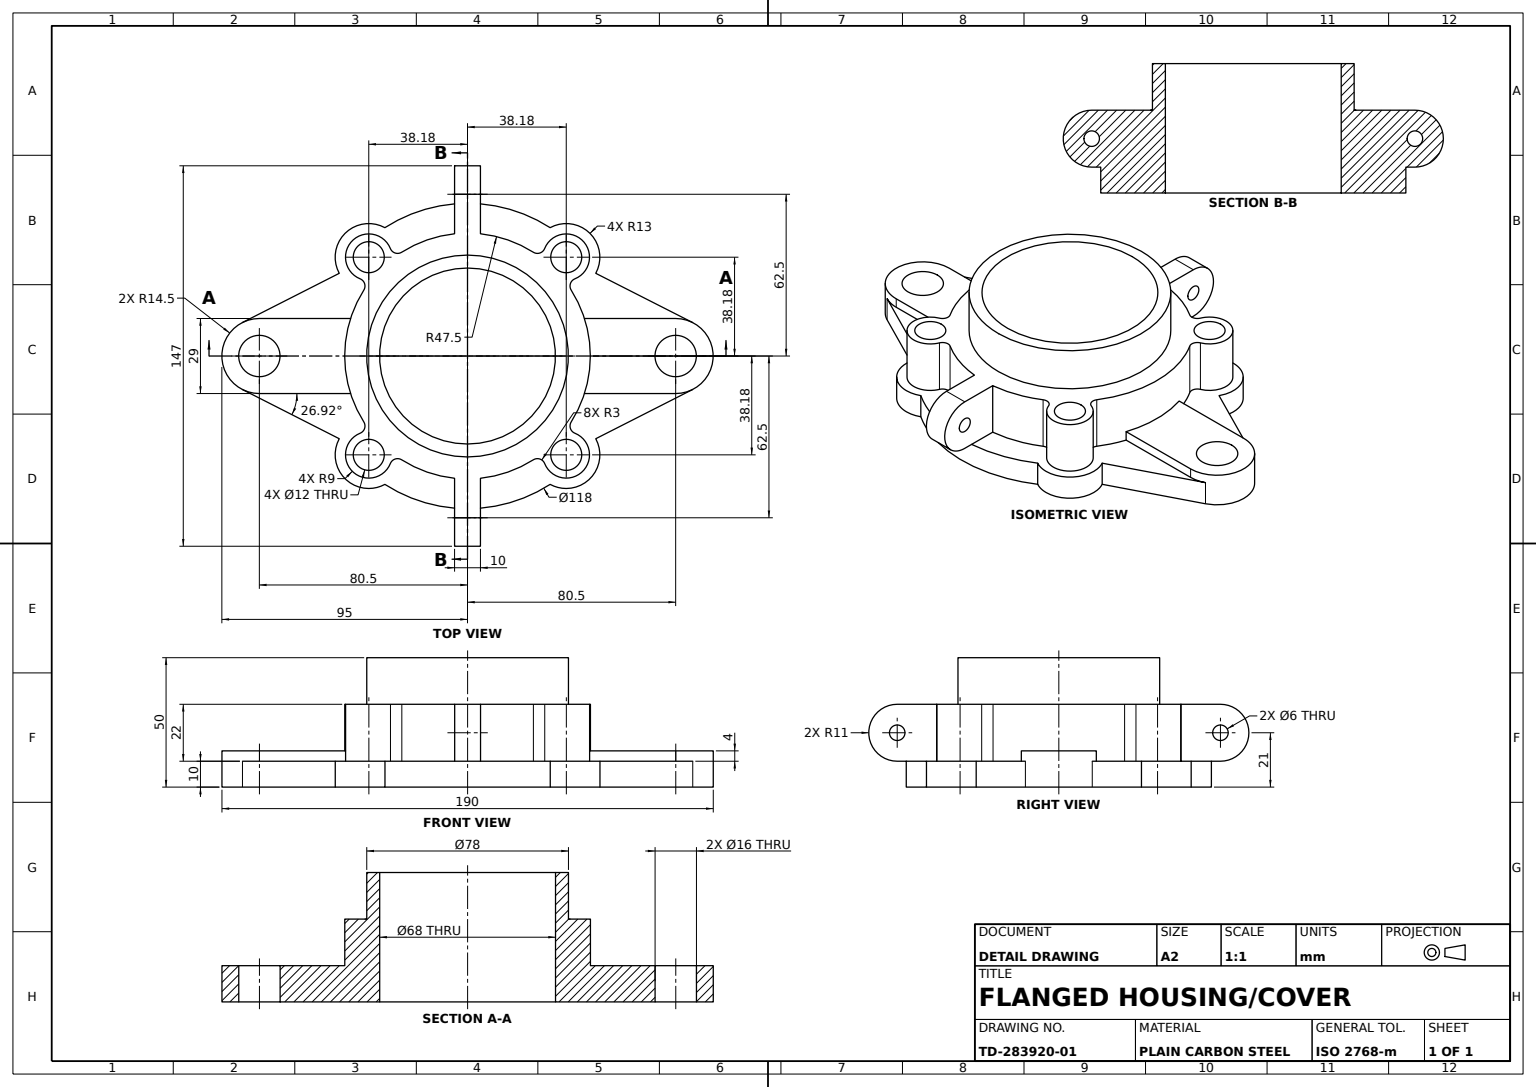
SolidWorks part; units mm, degrees
material "Plain Carbon Steel"
ref_plane "Front Plane" through (0, 0, 0) normal (0, 0, 1) x (1, 0, 0)
ref_plane "Top Plane" through (0, 0, 0) normal (0, 1, 0) x (1, 0, 0)
ref_plane "Right Plane" through (0, 0, 0) normal (1, 0, 0) x (0, 0, -1)
sketch "Base Flange Sketch" plane through (0, 0, 0) normal (0, 1, 0) x (1, 0, 0)
  circle A0 centre (0, 0) radius 59
  dimension "D1" = 118
extrude "Base Flange Ø118" add sketch "Base Flange Sketch" along normal blind 10
sketch "Flange Lobes Sketch" plane through (0, 10, 0) normal (0, 1, 0) x (1, 0, 0)
  line L0 (-54, 0) -> (54, 0) construction
  line L1 (54, 0) -> (0, 0) construction
  line L2 (0, 0) -> (0, 54) construction
  line L3 (0, 54) -> (0, -54) construction
  line L4 (0, -54) -> (0, 0) construction
  line L5 (0, 0) -> (38.1838, -38.1838) construction
  line L6 (38.1838, -38.1838) -> (-38.1838, 38.1838) construction
  line L7 (-38.1838, 38.1838) -> (0, 0) construction
  line L8 (0, 0) -> (-38.1838, -38.1838) construction
  line L9 (-38.1838, -38.1838) -> (38.1838, 38.1838) construction
  circle A0 centre (0, 0) radius 54 construction
  circle A1 centre (-38.1838, 38.1838) radius 13
  circle A3 centre (38.1838, 38.1838) radius 13
  circle A5 centre (38.1838, -38.1838) radius 13
  circle A6 centre (-38.1838, -38.1838) radius 13
  dimension "D1" = 108
  dimension "D6" = 26
  dimension "D7" = 26
  dimension "D8" = 26
  dimension "D9" = 26
  dimension "D2" = 45
  dimension "D3" = 45
  dimension "D4" = 45
  dimension "D5" = 45
extrude "Flange Lobes" add sketch "Flange Lobes Sketch" against normal blind 10
sketch "Hub and Bosses Sketch" plane through (0, 10, 0) normal (0, 1, 0) x (1, 0, 0)
  line L0 (-47.3762, 47.3762) -> (47.3762, -47.3762) construction
  line L1 (47.3762, -47.3762) -> (0, 0) construction
  line L2 (0, 0) -> (47.3762, 47.3762) construction
  line L3 (47.3762, 47.3762) -> (-47.3762, -47.3762) construction
  arc A0 (-40.1141, 25.4383) -> (-40.1141, -25.4383) centre (0, 0) ccw
  arc A1 (-31.9573, 49.5957) -> (-49.5957, 31.9573) centre (-38.1838, 38.1838) ccw construction
  arc A2 (31.9573, -49.5957) -> (49.5957, -31.9573) centre (38.1838, -38.1838) ccw construction
  arc A3 (49.5957, 31.9573) -> (31.9573, 49.5957) centre (38.1838, 38.1838) ccw construction
  arc A4 (-49.5957, -31.9573) -> (-31.9573, -49.5957) centre (-38.1838, -38.1838) ccw construction
  arc A5 (-29.8296, 41.5317) -> (-41.5317, 29.8296) centre (-38.1838, 38.1838) ccw
  arc A6 (41.5317, 29.8296) -> (29.8296, 41.5317) centre (38.1838, 38.1838) ccw
  arc A7 (29.8296, -41.5317) -> (41.5317, -29.8296) centre (38.1838, -38.1838) ccw
  arc A8 (-41.5317, -29.8296) -> (-29.8296, -41.5317) centre (-38.1838, -38.1838) ccw
  circle A9 centre (-38.1838, 38.1838) radius 6
  circle A10 centre (38.1838, 38.1838) radius 6
  circle A11 centre (38.1838, -38.1838) radius 6
  circle A12 centre (-38.1838, -38.1838) radius 6
  arc A13 (25.4383, 40.1141) -> (-25.4383, 40.1141) centre (0, 0) ccw
  arc A14 (40.1141, -25.4383) -> (40.1141, 25.4383) centre (0, 0) ccw
  arc A15 (-25.4383, -40.1141) -> (25.4383, -40.1141) centre (0, 0) ccw
  arc A16 (-40.1141, 25.4383) -> (-41.5317, 29.8296) centre (-42.6476, 27.0449) ccw
  arc A17 (-40.1141, -25.4383) -> (-41.5317, -29.8296) centre (-42.6476, -27.0449) cw
  arc A18 (-29.8296, -41.5317) -> (-25.4383, -40.1141) centre (-27.0449, -42.6476) cw
  arc A19 (25.4383, -40.1141) -> (29.8296, -41.5317) centre (27.0449, -42.6476) cw
  arc A20 (41.5317, -29.8296) -> (40.1141, -25.4383) centre (42.6476, -27.0449) cw
  arc A21 (40.1141, 25.4383) -> (41.5317, 29.8296) centre (42.6476, 27.0449) cw
  arc A22 (29.8296, 41.5317) -> (25.4383, 40.1141) centre (27.0449, 42.6476) cw
  arc A23 (-25.4383, 40.1141) -> (-29.8296, 41.5317) centre (-27.0449, 42.6476) cw
  point P48 (37.4544, -29.2134)
  dimension "D1" = 95
  dimension "D2" = 18
  dimension "D3" = 18
  dimension "D4" = 18
  dimension "D5" = 18
  dimension "D6" = 12
  dimension "D7" = 12
  dimension "D8" = 12
  dimension "D9" = 12
  dimension "D10" = 3
  dimension "D11" = 3
extrude "Hub with Bolt Bosses" add sketch "Hub and Bosses Sketch" along normal blind 22
sketch "Pipe Collar Sketch" plane through (0, 32, 0) normal (0, 1, 0) x (1, 0, 0)
  circle A0 centre (0, 0) radius 39
  circle A1 centre (0, 0) radius 34
  dimension "D1" = 78
  dimension "D2" = 68
extrude "Pipe Collar Ø78" add sketch "Pipe Collar Sketch" along normal blind 18
sketch "Side Lugs Sketch" plane through (0, 10, 0) normal (0, 1, 0) x (1, 0, 0)
  line L1 (-5, -47.2361) -> (-5, -62.5)
  line L2 (-5, -62.5) -> (5, -62.5)
  line L3 (5, -62.5) -> (5, -47.2361)
  line L5 (-5, 47.2361) -> (-5, 62.5)
  line L6 (-5, 62.5) -> (5, 62.5)
  line L7 (5, 62.5) -> (5, 47.2361)
  arc A0 (5, 47.2361) -> (-5, 47.2361) centre (0, 0) ccw
  arc A1 (-5, -47.2361) -> (5, -47.2361) centre (0, 0) ccw
  dimension "D1" = 47.5
  dimension "D2" = 36.5317
  dimension "D3" = 32.6704
extrude "Side Lugs" add sketch "Side Lugs Sketch" along normal blind 22
sketch "Lug Gusset A Sketch" plane through (5, 0, 0) normal (1, 0, 0) x (0, 0, -1)
  line L0 (-62.5, 32) -> (-62.5, 10) construction
  line L1 (-62.5, 32) -> (-47.2361, 32)
  line L2 (-47.2361, 32) -> (-47.2361, 10) construction
  line L3 (-62.5, 32) -> (-47.2361, 32) construction
  line L4 (-47.2361, 32) -> (-47.1838, 10)
  line L5 (-47.1838, 32) -> (-47.1838, 10) construction
  line L6 (-47.1838, 10) -> (-62.5, 10)
  arc A0 (-62.5, 32) -> (-62.5, 10) centre (-62.5, 21) ccw
  circle A1 centre (-62.5, 21) radius 3
  dimension "D1" = 6
extrude "Lug Gusset A" add sketch "Lug Gusset A Sketch" against normal blind 10
sketch "Lug Hole A Sketch" plane through (5, 0, 0) normal (1, 0, 0) x (0, 0, -1)
  circle A0 centre (-62.5, 21) radius 3
  dimension "D1" = 6
extrude "Lug Hole A" cut sketch "Lug Hole A Sketch" against normal blind 10
sketch "Lug Gusset B Sketch" plane through (5, 0, 0) normal (1, 0, 0) x (0, 0, -1)
  line L0 (62.5, 32) -> (62.5, 10) construction
  line L1 (62.5, 32) -> (47.1838, 32)
  line L2 (47.1838, 32) -> (47.2361, 10)
  line L3 (51.1838, 10) -> (31.9573, 10) construction
  line L4 (47.2361, 32) -> (47.2361, 10) construction
  line L5 (47.2361, 10) -> (62.5, 10)
  arc A0 (62.5, 10) -> (62.5, 32) centre (62.5, 21) ccw
  circle A1 centre (62.5, 21) radius 3
  dimension "D1" = 6
extrude "Lug Gusset B" add sketch "Lug Gusset B Sketch" against normal blind 10
sketch "Lug Hole B Sketch" plane through (5, 0, 0) normal (1, 0, 0) x (0, 0, -1)
  line L0 (62.5, 24) -> (62.5, 18) construction
  circle A0 centre (62.5, 21) radius 3
  dimension "D1" = 6
extrude "Lug Hole B" cut sketch "Lug Hole B Sketch" against normal blind 10
sketch "Mounting Ears Sketch" plane through (0, 0, 0) normal (0, 1, 0) x (1, 0, 0)
  line L0 (-80.5, 0) -> (80.5, 0) construction
  line L1 (-87.0656, 12.9284) -> (-49.5957, 31.9573)
  line L2 (-87.0656, -12.9284) -> (-49.5957, -31.9573)
  line L3 (87.0656, 12.9284) -> (49.5957, 31.9573)
  line L4 (87.0656, -12.9284) -> (49.5957, -31.9573)
  arc A0 (-87.0656, 12.9284) -> (-87.0656, -12.9284) centre (-80.5, 0) ccw
  circle A1 centre (-80.5, 0) radius 8
  arc A7 (87.0656, -12.9284) -> (87.0656, 12.9284) centre (80.5, 0) ccw
  circle A8 centre (80.5, 0) radius 8
  arc A9 (49.5957, -31.9573) -> (49.5957, 31.9573) centre (0, 0) ccw
  arc A10 (-49.5957, 31.9573) -> (-49.5957, -31.9573) centre (0, 0) ccw
  dimension "D3" = 29
  dimension "D4" = 16
  dimension "D5" = 29
  dimension "D6" = 16
  dimension "D7" = 59
  dimension "D1" = 80.5
  dimension "D2" = 80.5
  dimension "D8" = 6.5656
  dimension "D9" = 37.47
extrude "Mounting Ears" add sketch "Mounting Ears Sketch" along normal blind 10
sketch "Ear Rib A Sketch" plane through (0, 10, 0) normal (0, 1, 0) x (1, 0, 0)
  line L0 (-80.5, 14.5) -> (-45.2327, 14.5)
  line L1 (-80.5, -14.5) -> (-45.2327, -14.5)
  arc A6 (-80.5, 14.5) -> (-80.5, -14.5) centre (-80.5, 0) ccw
  arc A7 (-40.1141, 25.4383) -> (-40.1141, -25.4383) centre (0, 0) ccw construction
  arc A8 (-45.2327, 14.5) -> (-45.2327, -14.5) centre (0, 0) ccw
  circle A9 centre (-80.5, 0) radius 8 construction
  circle A10 centre (-80.5, 0) radius 8
  dimension "D1" = 14.5
extrude "Ear Rib A" add sketch "Ear Rib A Sketch" along normal blind 4
sketch "Ear Rib B Sketch" plane through (0, 10, 0) normal (0, 1, 0) x (1, 0, 0)
  line L0 (80.5, 14.5) -> (45.2327, 14.5)
  line L1 (80.5, -14.5) -> (45.2327, -14.5)
  arc A0 (80.5, -14.5) -> (80.5, 14.5) centre (80.5, 0) ccw
  arc A1 (40.1141, -25.4383) -> (40.1141, 25.4383) centre (0, 0) ccw construction
  arc A2 (45.2327, -14.5) -> (45.2327, 14.5) centre (0, 0) ccw
  circle A3 centre (80.5, 0) radius 8 construction
  circle A4 centre (80.5, 0) radius 8
  dimension "D1" = 14.5
extrude "Ear Rib B" add sketch "Ear Rib B Sketch" along normal blind 4
sketch "Side Relief Cut Sketch" plane through (0, 32, 0) normal (0, 1, 0) x (1, 0, 0)
  circle A0 centre (-38.1838, 38.1838) radius 6
  circle A1 centre (38.1838, 38.1838) radius 6
  circle A2 centre (38.1838, -38.1838) radius 6
  circle A3 centre (-38.1838, -38.1838) radius 6
  dimension "D1" = 12
extrude "Side Relief Cut" cut sketch "Side Relief Cut Sketch" against normal up to next
sketch "Pipe Bore Sketch" plane through (0, 32, 0) normal (0, 1, 0) x (1, 0, 0)
  circle A0 centre (0, 0) radius 34
  dimension "D1" = 68
extrude "Pipe Bore" cut sketch "Pipe Bore Sketch" against normal up to next
